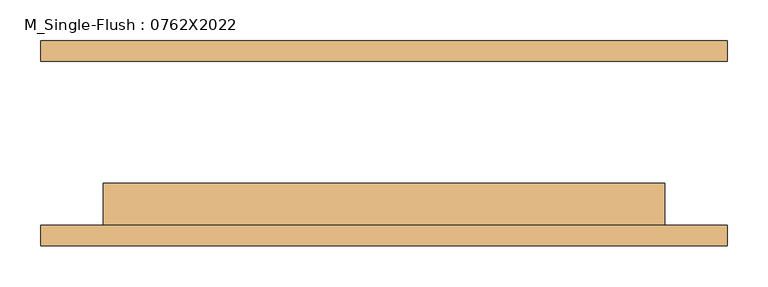
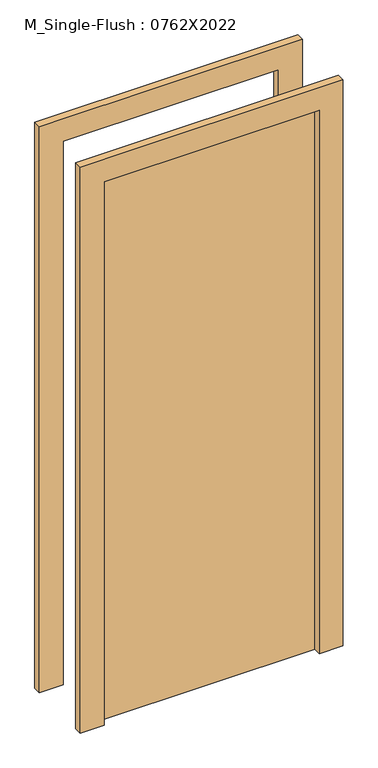
"""IFC4 building model written with IfcOpenShell, lengths in millimetres: door geometry, M_Single-Flush : 0762X2022."""

from ifc_helpers import new_model, si_unit, frame, origin, origin_with_axes, place, context, project, spatial, polyline, outline, extrude, source, transform, mapped, element, save


def m_single_flush_0762x2022_6401452f(model_context):
    return source(origin(), model_context, "Body", "SweptSolid", [
        extrude(outline(polyline([(1904.8, -418.9), (0.0, -418.9), (0.0, -342.9), (1828.8, -342.9), (1828.8, 342.9), (0.0, 342.9), (0.0, 418.9), (1904.8, 418.9), (1904.8, -418.9)])), frame((0.0, -125.0, 0.0), z_axis=(0.0, 1.0, 0.0), x_axis=(0.0, 0.0, 1.0)), (0.0, 0.0, 1.0), 25.0),
        extrude(outline(polyline([(1904.8, 418.9), (1904.8, -418.9), (0.0, -418.9), (0.0, -342.9), (1828.8, -342.9), (1828.8, 342.9), (0.0, 342.9), (0.0, 418.9), (1904.8, 418.9)])), frame((0.0, 100.0, 0.0), z_axis=(0.0, 1.0, 0.0), x_axis=(0.0, 0.0, 1.0)), (0.0, 0.0, 1.0), 25.0),
        extrude(outline(polyline([(342.9, -49.0), (342.9, -100.0), (-342.9, -100.0), (-342.9, -49.0), (342.9, -49.0)])), origin_with_axes(), (0.0, 0.0, 1.0), 1828.8),
    ])


if __name__ == "__main__":
    model = new_model("IFC4")
    model_context = context("Model", 3, world=origin())
    ifc_project = project(units=[si_unit("LENGTHUNIT", "METRE", prefix="MILLI")], contexts=[model_context])
    site = spatial("IfcSite", under=ifc_project)
    building = spatial("IfcBuilding", under=site)
    placement = place(None, origin())
    m_single_flush_0762x2022_shape = m_single_flush_0762x2022_6401452f(model_context)
    element("IfcDoor", 1, ObjectType="M_Single-Flush : 0762X2022", at=placement, inside=building, context=model_context, shape_type="MappedRepresentation", body=[
        mapped(m_single_flush_0762x2022_shape, transform((0.0, 0.0, 0.0), x_axis=(1.0, 0.0, 0.0), y_axis=(0.0, 1.0, 0.0), z_axis=(0.0, 0.0, 1.0))),
    ])
    save(model, "model.ifc")

# Revit data of these elements
# Type "M_Single-Flush : 0762X2022"
#   Type Mark = "22"
#   Thickness = 0' - 2.00787"
#   Height = 6' - 0"
#   Trim Projection Ext = 0' - 0.98425"
#   Trim Projection Int = 0' - 0.98425"
#   Trim Width = 0' - 2.99213"
#   Width = 2' - 3"
#   Door Material = Door - Panel
#   Frame Material = Door - Frame
#   Function = (empty or 0)
#   Wall Closure = (empty or 0)
# Element 1 (IfcDoor, "M_Single-Flush : 0762X2022")
#   Materials on its faces: "Door - Frame", "Door - Panel"
# Materials
#   "Door - Panel": class "Wood", colour RGB 114 82 51, transparency 0
#   "Door - Frame": colour RGB 153 76 43, transparency 0
